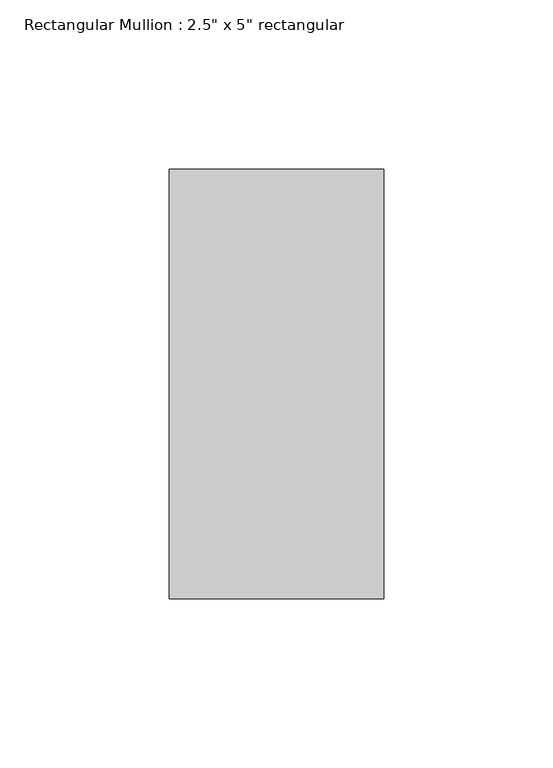
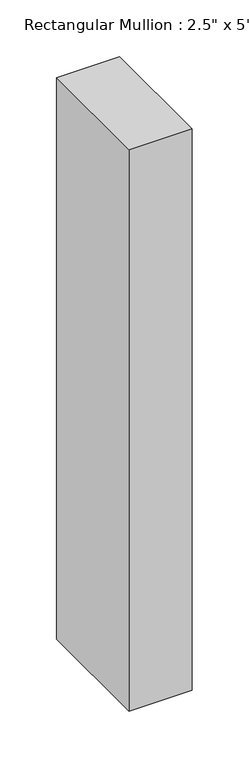
"""IFC4 building model written with IfcOpenShell, lengths in millimetres: member geometry."""

from ifc_helpers import new_model, si_unit, frame, origin, place, context, project, spatial, polyline, outline, extrude, source, transform, mapped, element, save


def member_576e3203(model_context):
    return source(origin(), model_context, "Body", "SweptSolid", [
        extrude(outline(polyline([(31.75, 63.5), (31.75, -63.5), (-31.75, -63.5), (-31.75, 63.5), (31.75, 63.5)])), frame((0.0, 0.0, -601.1333333), z_axis=(0.0, 0.0, 1.0), x_axis=(1.0, 0.0, 0.0)), (0.0, 0.0, 1.0), 601.1333333),
    ])


if __name__ == "__main__":
    model = new_model("IFC4")
    model_context = context("Model", 3, world=origin())
    ifc_project = project(units=[si_unit("LENGTHUNIT", "METRE", prefix="MILLI")], contexts=[model_context])
    site = spatial("IfcSite", under=ifc_project)
    building = spatial("IfcBuilding", under=site)
    placement = place(None, origin())
    member_shape = member_576e3203(model_context)
    element("IfcMember", 1, ObjectType="Rectangular Mullion : 2.5\" x 5\" rectangular", at=placement, inside=building, context=model_context, shape_type="MappedRepresentation", body=[
        mapped(member_shape, transform((0.0, 0.0, 0.0), x_axis=(1.0, 0.0, 0.0), y_axis=(0.0, 1.0, 0.0), z_axis=(0.0, 0.0, 1.0))),
    ])
    save(model, "model.ifc")

# Revit data of these elements
# Type "Rectangular Mullion : 2.5\" x 5\" rectangular"
#   built-in parameter 1007304 = 0.416667 (stored number, unit not read)
#   built-in parameter 1007301 = 0.104167 (stored number, unit not read)
#   built-in parameter 1007300 = 0.104167 (stored number, unit not read)
# Element 1 (IfcMember, "Rectangular Mullion : 2.5\" x 5\" rectangular")
#   Materials on its faces: "Aluminum"
# Materials
#   "Aluminum": class "Metal", colour RGB 247 247 247, transparency 0, Description = "Aluminum 6061", Cost = 0
